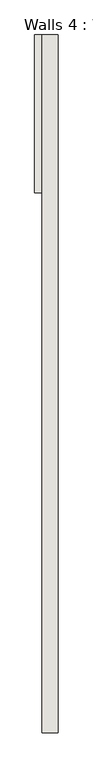
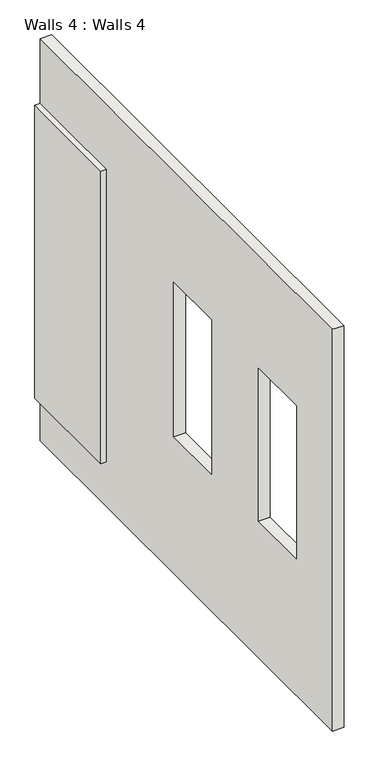
"""IFC4 building model written with IfcOpenShell, lengths in millimetres: wall geometry, Walls 4 : Walls 4."""

from ifc_helpers import new_model, si_unit, frame, origin, place, context, project, spatial, polyline, outline, extrude, source, transform, mapped, element, save


def walls_4_walls_4_3d1cd982(model_context):
    return source(origin(), model_context, "Body", "SweptSolid", [
        extrude(outline(polyline([(-11366.628584, 6697.1114178), (-11366.628584, 7763.9114178), (-11208.6620963, 7763.9114178), (-11208.6620963, 6697.1114178), (-11366.628584, 6697.1114178)])), frame((0.0, 0.0, 4095.8208602), z_axis=(0.0, 0.0, 1.0), x_axis=(1.0, 0.0, 0.0)), (0.0, 0.0, 1.0), 2884.5866319),
        extrude(outline(polyline([(3039.5114178, 7620.0), (7763.9114178, 7620.0), (7763.9114178, 3657.6), (3039.5114178, 3657.6), (3039.5114178, 7620.0)]), holes=[polyline([(4995.3114178, 6529.3782841), (4995.3114178, 5005.3782841), (5604.9114178, 5005.3782841), (5604.9114178, 6529.3782841), (4995.3114178, 6529.3782841)]), polyline([(3623.7114178, 6513.5923365), (3623.7114178, 5005.3782841), (4233.3114178, 5005.3782841), (4233.3114178, 6513.5923365), (3623.7114178, 6513.5923365)])]), frame((-11316.5075681, 0.0, 0.0), z_axis=(1.0, 0.0, 0.0), x_axis=(0.0, 1.0, 0.0)), (0.0, 0.0, 1.0), 107.8454718),
    ])


if __name__ == "__main__":
    model = new_model("IFC4")
    model_context = context("Model", 3, world=origin())
    ifc_project = project(units=[si_unit("LENGTHUNIT", "METRE", prefix="MILLI")], contexts=[model_context])
    site = spatial("IfcSite", under=ifc_project)
    building = spatial("IfcBuilding", under=site)
    placement = place(None, origin())
    walls_4_walls_4_shape = walls_4_walls_4_3d1cd982(model_context)
    element("IfcWall", 1, ObjectType="Walls 4 : Walls 4", at=placement, inside=building, context=model_context, shape_type="MappedRepresentation", body=[
        mapped(walls_4_walls_4_shape, transform((0.0, 0.0, 0.0), x_axis=(1.0, 0.0, 0.0), y_axis=(0.0, 1.0, 0.0), z_axis=(0.0, 0.0, 1.0))),
    ])
    save(model, "model.ifc")

# Revit data of these elements
# Element 1 (IfcWall, "Walls 4 : Walls 4")
#   Materials on its faces: "Default Wall"
# Materials
#   "Default Wall": colour RGB 128 128 128, transparency 0
